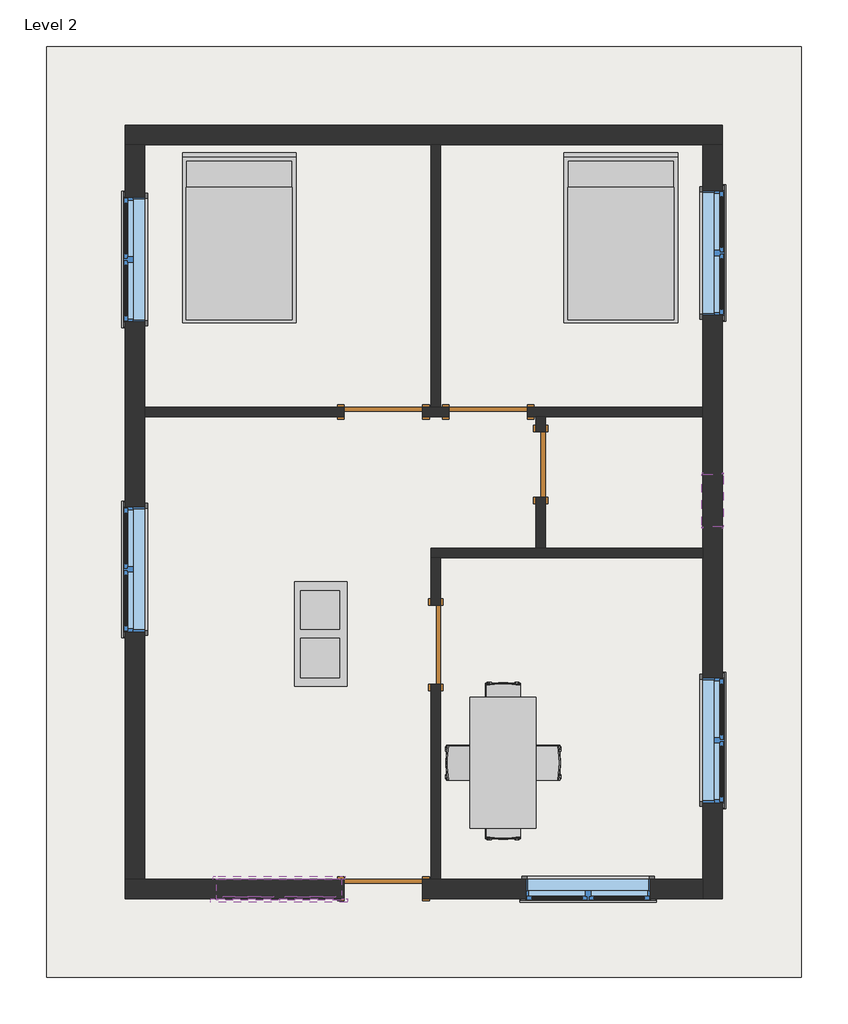
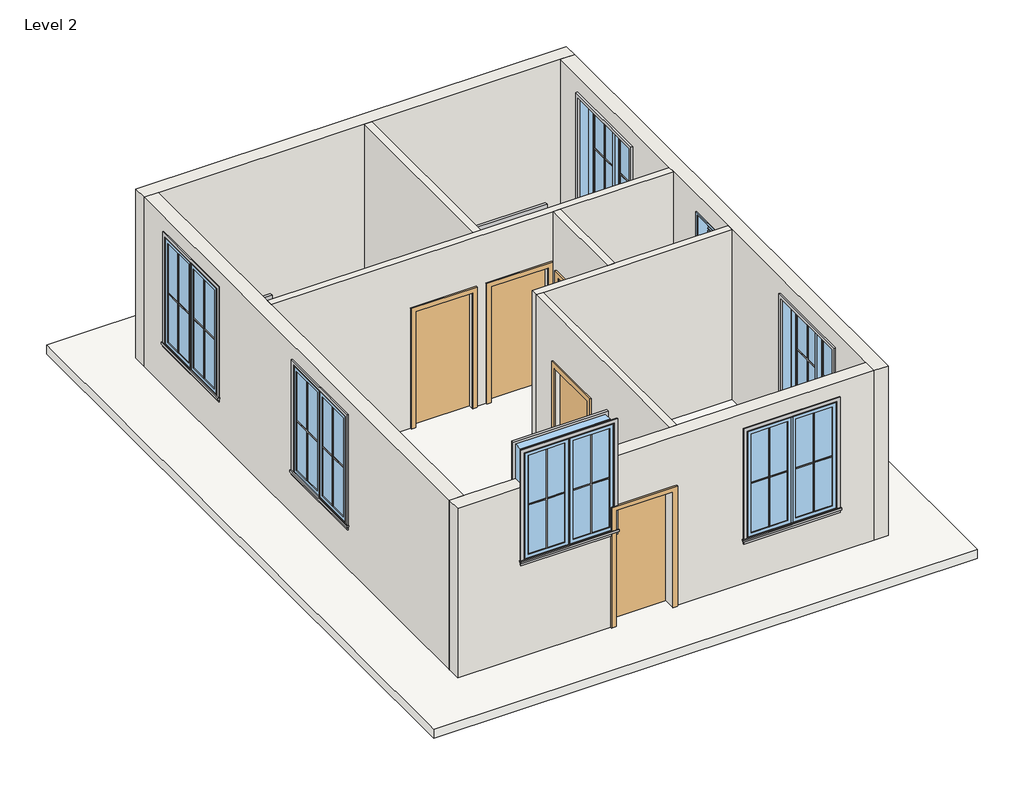
# One storey, incomplete: 25 proxies, 9 walls, 7 windows, 5 doors, 3 furniture elements, 1 roof.
"""IFC4 building model written with IfcOpenShell, lengths in millimetres."""

from ifc_helpers import new_model, si_unit, frame, origin, place, context, project, spatial, polyline, outline, extrude, faceted_brep, transform, mapped, element, save
from components import muntin_pattern_2x2_muntin_pattern_2x2_bff912c5, muntin_pattern_2x2_muntin_pattern_2x2_c2194282, trim_window_exterior_flat_with_sill_e04b3088, trim_window_interior_flat_picture_frame_2a7685fe, coffee_table_with_brass_mullions_11320_coffee_table_with_5962bef7, door_305aa2a5, door_e5f9f3c4, door_0ca8825f, door_f2b275c1, bed_17739_bed_17739_15c61121, dining_table_w_chairs_11374_0cdfc61b, window_9ac97e1a, window_f2d8fef0

model = new_model("IFC4")

# Units and contexts
model_context = context("Model", 3, world=origin())
ifc_project = project(units=[si_unit("LENGTHUNIT", "METRE", prefix="MILLI")], contexts=[model_context])

# Site, building, storey
site = spatial("IfcSite", under=ifc_project)
building = spatial("IfcBuilding", under=site)
storey = spatial("IfcBuildingStorey", under=building, Name="Level 2", Elevation=3048.0)

# Proxies
placement = place(None, origin())
muntin_pattern_2x2_muntin_pattern_2x2_shape = muntin_pattern_2x2_muntin_pattern_2x2_bff912c5(model_context)
element("IfcBuildingElementProxy", 1, Name="Muntin Pattern_2x2 : Muntin Pattern_2x2", ObjectType="Muntin Pattern_2x2 : Muntin Pattern_2x2", at=placement, inside=storey, context=model_context, shape_type="MappedRepresentation", body=[
    mapped(muntin_pattern_2x2_muntin_pattern_2x2_shape, transform((-4718.1437352, -1580.3188735, 4032.25), x_axis=(0.0, 1.0, 0.0), y_axis=(-1.0, 0.0, 0.0), z_axis=(0.0, 0.0, 1.0))),
])
element("IfcBuildingElementProxy", 2, Name="Muntin Pattern_2x2 : Muntin Pattern_2x2", ObjectType="Muntin Pattern_2x2 : Muntin Pattern_2x2", at=placement, inside=storey, context=model_context, shape_type="MappedRepresentation", body=[
    mapped(muntin_pattern_2x2_muntin_pattern_2x2_shape, transform((-2576.6062352, -5039.4813735, 4923.115521), x_axis=(-1.0, 0.0, 0.0), y_axis=(0.0, -1.0, 0.0), z_axis=(0.0, 0.0, 1.0))),
])
element("IfcBuildingElementProxy", 3, Name="Muntin Pattern_2x2 : Muntin Pattern_2x2", ObjectType="Muntin Pattern_2x2 : Muntin Pattern_2x2", at=placement, inside=storey, context=model_context, shape_type="MappedRepresentation", body=[
    mapped(muntin_pattern_2x2_muntin_pattern_2x2_shape, transform((1017.4937648, -5039.4813735, 4032.25), x_axis=(-1.0, 0.0, 0.0), y_axis=(0.0, -1.0, 0.0), z_axis=(0.0, 0.0, 1.0))),
])
element("IfcBuildingElementProxy", 4, Name="Muntin Pattern_2x2 : Muntin Pattern_2x2", ObjectType="Muntin Pattern_2x2 : Muntin Pattern_2x2", at=placement, inside=storey, context=model_context, shape_type="MappedRepresentation", body=[
    mapped(muntin_pattern_2x2_muntin_pattern_2x2_shape, transform((2209.7062648, -2847.1438735, 4032.25), x_axis=(0.0, -1.0, 0.0), y_axis=(1.0, 0.0, 0.0), z_axis=(0.0, 0.0, 1.0))),
])
element("IfcBuildingElementProxy", 5, Name="Muntin Pattern_2x2 : Muntin Pattern_2x2", ObjectType="Muntin Pattern_2x2 : Muntin Pattern_2x2", at=placement, inside=storey, context=model_context, shape_type="MappedRepresentation", body=[
    mapped(muntin_pattern_2x2_muntin_pattern_2x2_shape, transform((2209.7062648, 2817.0561265, 4032.25), x_axis=(0.0, -1.0, 0.0), y_axis=(1.0, 0.0, 0.0), z_axis=(0.0, 0.0, 1.0))),
])
element("IfcBuildingElementProxy", 6, Name="Muntin Pattern_2x2 : Muntin Pattern_2x2", ObjectType="Muntin Pattern_2x2 : Muntin Pattern_2x2", at=placement, inside=storey, context=model_context, shape_type="MappedRepresentation", body=[
    mapped(muntin_pattern_2x2_muntin_pattern_2x2_shape, transform((-4718.1437352, 2020.1311265, 4032.25), x_axis=(0.0, 1.0, 0.0), y_axis=(-1.0, 0.0, 0.0), z_axis=(0.0, 0.0, 1.0))),
])
muntin_pattern_2x2_muntin_pattern_2x2_2_shape = muntin_pattern_2x2_muntin_pattern_2x2_c2194282(model_context)
element("IfcBuildingElementProxy", 7, Name="Muntin Pattern_2x2 : Muntin Pattern_2x2", ObjectType="Muntin Pattern_2x2 : Muntin Pattern_2x2", at=placement, inside=storey, context=model_context, shape_type="MappedRepresentation", body=[
    mapped(muntin_pattern_2x2_muntin_pattern_2x2_2_shape, transform((-4718.1437352, -859.5938735, 4032.25), x_axis=(0.0, -1.0, 0.0), y_axis=(1.0, 0.0, 0.0), z_axis=(0.0, 0.0, 1.0))),
])
element("IfcBuildingElementProxy", 8, Name="Muntin Pattern_2x2 : Muntin Pattern_2x2", ObjectType="Muntin Pattern_2x2 : Muntin Pattern_2x2", at=placement, inside=storey, context=model_context, shape_type="MappedRepresentation", body=[
    mapped(muntin_pattern_2x2_muntin_pattern_2x2_2_shape, transform((-3297.3312352, -5039.4813735, 4923.115521), x_axis=(1.0, 0.0, 0.0), y_axis=(0.0, 1.0, 0.0), z_axis=(0.0, 0.0, 1.0))),
])
element("IfcBuildingElementProxy", 9, Name="Muntin Pattern_2x2 : Muntin Pattern_2x2", ObjectType="Muntin Pattern_2x2 : Muntin Pattern_2x2", at=placement, inside=storey, context=model_context, shape_type="MappedRepresentation", body=[
    mapped(muntin_pattern_2x2_muntin_pattern_2x2_2_shape, transform((296.7687648, -5039.4813735, 4032.25), x_axis=(1.0, 0.0, 0.0), y_axis=(0.0, 1.0, 0.0), z_axis=(0.0, 0.0, 1.0))),
])
element("IfcBuildingElementProxy", 10, Name="Muntin Pattern_2x2 : Muntin Pattern_2x2", ObjectType="Muntin Pattern_2x2 : Muntin Pattern_2x2", at=placement, inside=storey, context=model_context, shape_type="MappedRepresentation", body=[
    mapped(muntin_pattern_2x2_muntin_pattern_2x2_2_shape, transform((2209.7062648, -3567.8688735, 4032.25), x_axis=(0.0, 1.0, 0.0), y_axis=(-1.0, 0.0, 0.0), z_axis=(0.0, 0.0, 1.0))),
])
element("IfcBuildingElementProxy", 11, Name="Muntin Pattern_2x2 : Muntin Pattern_2x2", ObjectType="Muntin Pattern_2x2 : Muntin Pattern_2x2", at=placement, inside=storey, context=model_context, shape_type="MappedRepresentation", body=[
    mapped(muntin_pattern_2x2_muntin_pattern_2x2_2_shape, transform((2209.7062648, 2096.3311265, 4032.25), x_axis=(0.0, 1.0, 0.0), y_axis=(-1.0, 0.0, 0.0), z_axis=(0.0, 0.0, 1.0))),
])
element("IfcBuildingElementProxy", 12, Name="Muntin Pattern_2x2 : Muntin Pattern_2x2", ObjectType="Muntin Pattern_2x2 : Muntin Pattern_2x2", at=placement, inside=storey, context=model_context, shape_type="MappedRepresentation", body=[
    mapped(muntin_pattern_2x2_muntin_pattern_2x2_2_shape, transform((-4718.1437352, 2740.8561265, 4032.25), x_axis=(0.0, -1.0, 0.0), y_axis=(1.0, 0.0, 0.0), z_axis=(0.0, 0.0, 1.0))),
])
trim_window_exterior_flat_with_sill_shape = trim_window_exterior_flat_with_sill_e04b3088(model_context)
element("IfcBuildingElementProxy", 13, Name="Trim-Window-Exterior-Flat : with Sill", ObjectType="Trim-Window-Exterior-Flat : with Sill", at=placement, inside=storey, context=model_context, shape_type="MappedRepresentation", body=[
    mapped(trim_window_exterior_flat_with_sill_shape, transform((-4727.6687352, -1219.9563735, 5791.2), x_axis=(0.0, -1.0, 0.0), y_axis=(0.0, 0.0, 1.0), z_axis=(-1.0, 0.0, 0.0))),
])
element("IfcBuildingElementProxy", 14, Name="Trim-Window-Exterior-Flat : with Sill", ObjectType="Trim-Window-Exterior-Flat : with Sill", at=placement, inside=storey, context=model_context, shape_type="MappedRepresentation", body=[
    mapped(trim_window_exterior_flat_with_sill_shape, transform((-2936.9687352, -5049.0063735, 6682.065521), x_axis=(1.0, 0.0, 0.0), y_axis=(0.0, 0.0, 1.0), z_axis=(0.0, -1.0, 0.0))),
])
element("IfcBuildingElementProxy", 15, Name="Trim-Window-Exterior-Flat : with Sill", ObjectType="Trim-Window-Exterior-Flat : with Sill", at=placement, inside=storey, context=model_context, shape_type="MappedRepresentation", body=[
    mapped(trim_window_exterior_flat_with_sill_shape, transform((657.1312648, -5049.0063735, 5791.2), x_axis=(1.0, 0.0, 0.0), y_axis=(0.0, 0.0, 1.0), z_axis=(0.0, -1.0, 0.0))),
])
element("IfcBuildingElementProxy", 16, Name="Trim-Window-Exterior-Flat : with Sill", ObjectType="Trim-Window-Exterior-Flat : with Sill", at=placement, inside=storey, context=model_context, shape_type="MappedRepresentation", body=[
    mapped(trim_window_exterior_flat_with_sill_shape, transform((2219.2312648, -3207.5063735, 5791.2), x_axis=(0.0, 1.0, 0.0), y_axis=(0.0, 0.0, 1.0), z_axis=(1.0, 0.0, 0.0))),
])
element("IfcBuildingElementProxy", 17, Name="Trim-Window-Exterior-Flat : with Sill", ObjectType="Trim-Window-Exterior-Flat : with Sill", at=placement, inside=storey, context=model_context, shape_type="MappedRepresentation", body=[
    mapped(trim_window_exterior_flat_with_sill_shape, transform((2219.2312648, 2456.6936265, 5791.2), x_axis=(0.0, 1.0, 0.0), y_axis=(0.0, 0.0, 1.0), z_axis=(1.0, 0.0, 0.0))),
])
element("IfcBuildingElementProxy", 18, Name="Trim-Window-Exterior-Flat : with Sill", ObjectType="Trim-Window-Exterior-Flat : with Sill", at=placement, inside=storey, context=model_context, shape_type="MappedRepresentation", body=[
    mapped(trim_window_exterior_flat_with_sill_shape, transform((-4727.6687352, 2380.4936265, 5791.2), x_axis=(0.0, -1.0, 0.0), y_axis=(0.0, 0.0, 1.0), z_axis=(-1.0, 0.0, 0.0))),
])
trim_window_interior_flat_picture_frame_shape = trim_window_interior_flat_picture_frame_2a7685fe(model_context)
element("IfcBuildingElementProxy", 19, Name="Trim-Window-Interior-Flat : Picture Frame", ObjectType="Trim-Window-Interior-Flat : Picture Frame", at=placement, inside=storey, context=model_context, shape_type="MappedRepresentation", body=[
    mapped(trim_window_interior_flat_picture_frame_shape, transform((-4499.0687352, -1219.9563735, 5791.2), x_axis=(0.0, 1.0, 0.0), y_axis=(0.0, 0.0, 1.0), z_axis=(1.0, 0.0, 0.0))),
])
element("IfcBuildingElementProxy", 20, Name="Trim-Window-Interior-Flat : Picture Frame", ObjectType="Trim-Window-Interior-Flat : Picture Frame", at=placement, inside=storey, context=model_context, shape_type="MappedRepresentation", body=[
    mapped(trim_window_interior_flat_picture_frame_shape, transform((-2936.9687352, -4820.4063735, 6682.065521), x_axis=(-1.0, 0.0, 0.0), y_axis=(0.0, 0.0, 1.0), z_axis=(0.0, 1.0, 0.0))),
])
element("IfcBuildingElementProxy", 21, Name="Trim-Window-Interior-Flat : Picture Frame", ObjectType="Trim-Window-Interior-Flat : Picture Frame", at=placement, inside=storey, context=model_context, shape_type="MappedRepresentation", body=[
    mapped(trim_window_interior_flat_picture_frame_shape, transform((657.1312648, -4820.4063735, 5791.2), x_axis=(-1.0, 0.0, 0.0), y_axis=(0.0, 0.0, 1.0), z_axis=(0.0, 1.0, 0.0))),
])
element("IfcBuildingElementProxy", 22, Name="Trim-Window-Interior-Flat : Picture Frame", ObjectType="Trim-Window-Interior-Flat : Picture Frame", at=placement, inside=storey, context=model_context, shape_type="MappedRepresentation", body=[
    mapped(trim_window_interior_flat_picture_frame_shape, transform((1990.6312648, -3207.5063735, 5791.2), x_axis=(0.0, -1.0, 0.0), y_axis=(0.0, 0.0, 1.0), z_axis=(-1.0, 0.0, 0.0))),
])
element("IfcBuildingElementProxy", 23, Name="Trim-Window-Interior-Flat : Picture Frame", ObjectType="Trim-Window-Interior-Flat : Picture Frame", at=placement, inside=storey, context=model_context, shape_type="MappedRepresentation", body=[
    mapped(trim_window_interior_flat_picture_frame_shape, transform((1990.6312648, 2456.6936265, 5791.2), x_axis=(0.0, -1.0, 0.0), y_axis=(0.0, 0.0, 1.0), z_axis=(-1.0, 0.0, 0.0))),
])
element("IfcBuildingElementProxy", 24, Name="Trim-Window-Interior-Flat : Picture Frame", ObjectType="Trim-Window-Interior-Flat : Picture Frame", at=placement, inside=storey, context=model_context, shape_type="MappedRepresentation", body=[
    mapped(trim_window_interior_flat_picture_frame_shape, transform((-4499.0687352, 2380.4936265, 5791.2), x_axis=(0.0, 1.0, 0.0), y_axis=(0.0, 0.0, 1.0), z_axis=(1.0, 0.0, 0.0))),
])
coffee_table_with_brass_mullions_11320_coffee_table_with_shape = coffee_table_with_brass_mullions_11320_coffee_table_with_5962bef7(model_context)
element("IfcBuildingElementProxy", 25, Name="coffee_table_with_brass_mullions_11320 : coffee_table_with_brass_mullions_11320", ObjectType="coffee_table_with_brass_mullions_11320 : coffee_table_with_brass_mullions_11320", at=placement, inside=storey, context=model_context, shape_type="MappedRepresentation", body=[
    mapped(coffee_table_with_brass_mullions_11320_coffee_table_with_shape, transform((-2022.5687352, -1334.2563735, 3048.0), x_axis=(0.0, 1.0, 0.0), y_axis=(-1.0, 0.0, 0.0), z_axis=(0.0, 0.0, 1.0))),
])

# Doors
door_shape = door_305aa2a5(model_context)
element("IfcDoor", 26, ObjectType="Single-Flush : 36\" x 84\"", at=placement, inside=storey, context=model_context, shape_type="MappedRepresentation", body=[
    mapped(door_shape, transform((-1114.5187352, -2096.2563735, 3048.0), x_axis=(0.0, 1.0, 0.0), y_axis=(-1.0, 0.0, 0.0), z_axis=(0.0, 0.0, 1.0))),
])
element("IfcDoor", 27, ObjectType="Single-Flush : 36\" x 84\"", at=placement, inside=storey, context=model_context, shape_type="MappedRepresentation", body=[
    mapped(door_shape, transform((-1724.1187352, 608.8436265, 3048.0), x_axis=(-1.0, 0.0, 0.0), y_axis=(0.0, -1.0, 0.0), z_axis=(0.0, 0.0, 1.0))),
])
door_2_shape = door_e5f9f3c4(model_context)
element("IfcDoor", 28, ObjectType="Single-Flush : 36\" x 84\"", at=placement, inside=storey, context=model_context, shape_type="MappedRepresentation", body=[
    mapped(door_2_shape, transform((-504.9187352, 608.8436265, 3048.0), x_axis=(1.0, 0.0, 0.0), y_axis=(0.0, 1.0, 0.0), z_axis=(0.0, 0.0, 1.0))),
])
door_3_shape = door_0ca8825f(model_context)
element("IfcDoor", 29, ObjectType="Single-Flush : 36\" x 84\"", at=placement, inside=storey, context=model_context, shape_type="MappedRepresentation", body=[
    mapped(door_3_shape, transform((-1724.1187352, -4934.7063735, 3048.0), x_axis=(1.0, 0.0, 0.0), y_axis=(0.0, 1.0, 0.0), z_axis=(0.0, 0.0, 1.0))),
])
door_4_shape = door_f2b275c1(model_context)
element("IfcDoor", 30, ObjectType="Single-Flush : DOOR 2'6\"", at=placement, inside=storey, context=model_context, shape_type="MappedRepresentation", body=[
    mapped(door_4_shape, transform((104.6812648, -0.7563735, 3048.0), x_axis=(0.0, 1.0, 0.0), y_axis=(-1.0, 0.0, 0.0), z_axis=(0.0, 0.0, 1.0))),
])

# Furniture
bed_17739_bed_17739_shape = bed_17739_bed_17739_15c61121(model_context)
element("IfcFurniture", 31, ObjectType="Bed_17739 : Bed_17739", at=placement, inside=storey, context=model_context, shape_type="MappedRepresentation", body=[
    mapped(bed_17739_bed_17739_shape, transform((-3400.5187352, 2609.0936265, 3048.0), x_axis=(1.0, 0.0, 0.0), y_axis=(0.0, 1.0, 0.0), z_axis=(0.0, 0.0, 1.0))),
])
element("IfcFurniture", 32, ObjectType="Bed_17739 : Bed_17739", at=placement, inside=storey, context=model_context, shape_type="MappedRepresentation", body=[
    mapped(bed_17739_bed_17739_shape, transform((1038.1312648, 2609.0936265, 3048.0), x_axis=(1.0, 0.0, 0.0), y_axis=(0.0, 1.0, 0.0), z_axis=(0.0, 0.0, 1.0))),
])
dining_table_w_chairs_11374_shape = dining_table_w_chairs_11374_0cdfc61b(model_context)
element("IfcFurniture", 33, ObjectType="Dining_Table_w_Chairs_11374", at=placement, inside=storey, context=model_context, shape_type="MappedRepresentation", body=[
    mapped(dining_table_w_chairs_11374_shape, transform((-238.2576574, -3486.1221401, 3048.0), x_axis=(0.0, 1.0, 0.0), y_axis=(-1.0, 0.0, 0.0), z_axis=(0.0, 0.0, 1.0))),
])

# Roof
element("IfcRoof", 34, ObjectType="ROOF 6\"", at=placement, inside=storey, context=model_context, shape_type="SweptSolid", body=[
    extrude(outline(polyline([(-5642.0687352, 4856.9936265), (3133.6312648, 4856.9936265), (3133.6312648, -5963.4063735), (-5642.0687352, -5963.4063735), (-5642.0687352, 4856.9936265)])), frame((0.0, 0.0, 3048.0), z_axis=(0.0, 0.0, 1.0), x_axis=(1.0, 0.0, 0.0)), (0.0, 0.0, 1.0), 152.4),
])

# Walls
element("IfcWall", 35, ObjectType="WALL 4.5\"", at=placement, inside=storey, context=model_context, shape_type="Brep", body=[
    faceted_brep([(-4499.0687352, 551.6936265, 3048.0), (-2181.3187352, 551.6936265, 3048.0), (-2181.3187352, 551.6936265, 5181.6), (-1266.9187352, 551.6936265, 5181.6), (-1266.9187352, 551.6936265, 3048.0), (-962.1187352, 551.6936265, 3048.0), (-962.1187352, 551.6936265, 5181.6), (-47.7187352, 551.6936265, 5181.6), (-47.7187352, 551.6936265, 3048.0), (47.5312648, 551.6936265, 3048.0), (161.8312648, 551.6936265, 3048.0), (1990.6312648, 551.6936265, 3048.0), (1990.6312648, 551.6936265, 6096.0), (161.8312648, 551.6936265, 6096.0), (47.5312648, 551.6936265, 6096.0), (-4499.0687352, 551.6936265, 6096.0), (-2181.3187352, 665.9936265, 5181.6), (-2181.3187352, 665.9936265, 3048.0), (-4499.0687352, 665.9936265, 3048.0), (-4499.0687352, 665.9936265, 6096.0), (-1171.6687352, 665.9936265, 6096.0), (-1057.3687352, 665.9936265, 6096.0), (1990.6312648, 665.9936265, 6096.0), (1990.6312648, 665.9936265, 3048.0), (-47.7187352, 665.9936265, 3048.0), (-47.7187352, 665.9936265, 5181.6), (-962.1187352, 665.9936265, 5181.6), (-962.1187352, 665.9936265, 3048.0), (-1057.3687352, 665.9936265, 3048.0), (-1171.6687352, 665.9936265, 3048.0), (-1266.9187352, 665.9936265, 3048.0), (-1266.9187352, 665.9936265, 5181.6)], [[[0, 1, 2, 3, 4, 5, 6, 7, 8, 9, 10, 11, 12, 13, 14, 15]], [[16, 17, 18, 19, 20, 21, 22, 23, 24, 25, 26, 27, 28, 29, 30, 31]], [[11, 10, 9, 8, 24, 23]], [[18, 17, 1, 0]], [[30, 29, 28, 27, 5, 4]], [[12, 11, 23, 22]], [[0, 15, 19, 18]], [[25, 24, 8, 7]], [[26, 25, 7, 6]], [[27, 26, 6, 5]], [[2, 1, 17, 16]], [[3, 2, 16, 31]], [[4, 3, 31, 30]], [[15, 14, 13, 12, 22, 21, 20, 19]]]),
])
element("IfcWall", 36, ObjectType="WALL 4.5\"", at=placement, inside=storey, context=model_context, shape_type="SweptSolid", body=[
    extrude(outline(polyline([(-1057.3687352, 3713.9936265), (-1057.3687352, 665.9936265), (-1171.6687352, 665.9936265), (-1171.6687352, 3713.9936265), (-1057.3687352, 3713.9936265)])), frame((0.0, 0.0, 3048.0), z_axis=(0.0, 0.0, 1.0), x_axis=(1.0, 0.0, 0.0)), (0.0, 0.0, 1.0), 3048.0),
])
element("IfcWall", 37, ObjectType="WALL 4.5\"", at=placement, inside=storey, context=model_context, shape_type="Brep", body=[
    faceted_brep([(1990.6312648, -972.3063735, 3048.0), (161.8312648, -972.3063735, 3048.0), (47.5312648, -972.3063735, 3048.0), (-1171.6687352, -972.3063735, 3048.0), (-1171.6687352, -972.3063735, 6096.0), (47.5312648, -972.3063735, 6096.0), (161.8312648, -972.3063735, 6096.0), (1990.6312648, -972.3063735, 6096.0), (1990.6312648, -1086.6063735, 3048.0), (1990.6312648, -1086.6063735, 6096.0), (-1057.3687352, -1086.6063735, 6096.0), (-1171.6687352, -1086.6063735, 6096.0), (-1171.6687352, -1086.6063735, 3048.0), (-1057.3687352, -1086.6063735, 3048.0)], [[[0, 1, 2, 3, 4, 5, 6, 7]], [[8, 9, 10, 11, 12, 13]], [[3, 2, 1, 0, 8, 13, 12]], [[0, 7, 9, 8]], [[4, 3, 12, 11]], [[7, 6, 5, 4, 11, 10, 9]]]),
])
element("IfcWall", 38, ObjectType="WALL 4.5\"", at=placement, inside=storey, context=model_context, shape_type="SweptSolid", body=[
    extrude(outline(polyline([(-1086.6063735, 3048.0), (-1639.0563735, 3048.0), (-1639.0563735, 5181.6), (-2553.4563735, 5181.6), (-2553.4563735, 3048.0), (-4820.4063735, 3048.0), (-4820.4063735, 6096.0), (-1086.6063735, 6096.0), (-1086.6063735, 3048.0)])), frame((-1171.6687352, 0.0, 0.0), z_axis=(1.0, 0.0, 0.0), x_axis=(0.0, 1.0, 0.0)), (0.0, 0.0, 1.0), 114.3),
])
element("IfcWall", 39, ObjectType="WALL 4.5\"", at=placement, inside=storey, context=model_context, shape_type="SweptSolid", body=[
    extrude(outline(polyline([(551.6936265, 3048.0), (380.2436265, 3048.0), (380.2436265, 5080.0), (-381.7563735, 5080.0), (-381.7563735, 3048.0), (-972.3063735, 3048.0), (-972.3063735, 6096.0), (551.6936265, 6096.0), (551.6936265, 3048.0)])), frame((47.5312648, 0.0, 0.0), z_axis=(1.0, 0.0, 0.0), x_axis=(0.0, 1.0, 0.0)), (0.0, 0.0, 1.0), 114.3),
])
element("IfcWall", 40, ObjectType="WALL 9\"", at=placement, inside=storey, context=model_context, shape_type="Brep", body=[
    faceted_brep([(-4727.6687352, 3713.9936265, 3048.0), (-4499.0687352, 3713.9936265, 3048.0), (-1171.6687352, 3713.9936265, 3048.0), (-1057.3687352, 3713.9936265, 3048.0), (1990.6312648, 3713.9936265, 3048.0), (2219.2312648, 3713.9936265, 3048.0), (2219.2312648, 3713.9936265, 6096.0), (1990.6312648, 3713.9936265, 6096.0), (-1057.3687352, 3713.9936265, 6096.0), (-1171.6687352, 3713.9936265, 6096.0), (-4499.0687352, 3713.9936265, 6096.0), (-4727.6687352, 3713.9936265, 6096.0), (-4727.6687352, 3942.5936265, 3048.0), (-4727.6687352, 3942.5936265, 6096.0), (2219.2312648, 3942.5936265, 6096.0), (2219.2312648, 3942.5936265, 3048.0)], [[[0, 1, 2, 3, 4, 5, 6, 7, 8, 9, 10, 11]], [[12, 13, 14, 15]], [[5, 4, 3, 2, 1, 0, 12, 15]], [[6, 5, 15, 14]], [[0, 11, 13, 12]], [[11, 10, 9, 8, 7, 6, 14, 13]]]),
])
element("IfcWall", 41, ObjectType="WALL 9\"", at=placement, inside=storey, context=model_context, shape_type="Brep", body=[
    faceted_brep([(1990.6312648, 3713.9936265, 3048.0), (1990.6312648, 665.9936265, 3048.0), (1990.6312648, 551.6936265, 3048.0), (1990.6312648, -972.3063735, 3048.0), (1990.6312648, -1086.6063735, 3048.0), (1990.6312648, -4820.4063735, 3048.0), (1990.6312648, -5049.0063735, 3048.0), (1990.6312648, -5049.0063735, 6096.0), (1990.6312648, -4820.4063735, 6096.0), (1990.6312648, -1086.6063735, 6096.0), (1990.6312648, -972.3063735, 6096.0), (1990.6312648, 551.6936265, 6096.0), (1990.6312648, 665.9936265, 6096.0), (1990.6312648, 3713.9936265, 6096.0), (1990.6312648, -3931.4063735, 5791.2), (1990.6312648, -3931.4063735, 3962.4), (1990.6312648, -2483.6063735, 3962.4), (1990.6312648, -2483.6063735, 5791.2), (1990.6312648, 1732.7936265, 5791.2), (1990.6312648, 1732.7936265, 3962.4), (1990.6312648, 3180.5936265, 3962.4), (1990.6312648, 3180.5936265, 5791.2), (1990.6312648, -115.0563735, 5791.2), (1990.6312648, -724.6563735, 5791.2), (1990.6312648, -724.6563735, 5181.6), (1990.6312648, -115.0563735, 5181.6), (2219.2312648, 3713.9936265, 3048.0), (2219.2312648, 3713.9936265, 6096.0), (2219.2312648, -5049.0063735, 6096.0), (2219.2312648, -5049.0063735, 3048.0), (2219.2312648, -3931.4063735, 5791.2), (2219.2312648, -2483.6063735, 5791.2), (2219.2312648, -2483.6063735, 3962.4), (2219.2312648, -3931.4063735, 3962.4), (2219.2312648, 1732.7936265, 5791.2), (2219.2312648, 3180.5936265, 5791.2), (2219.2312648, 3180.5936265, 3962.4), (2219.2312648, 1732.7936265, 3962.4), (2219.2312648, -115.0563735, 5791.2), (2219.2312648, -115.0563735, 5181.6), (2219.2312648, -724.6563735, 5181.6), (2219.2312648, -724.6563735, 5791.2)], [[[0, 1, 2, 3, 4, 5, 6, 7, 8, 9, 10, 11, 12, 13], [14, 15, 16, 17], [18, 19, 20, 21], [22, 23, 24, 25]], [[26, 27, 28, 29], [30, 31, 32, 33], [34, 35, 36, 37], [38, 39, 40, 41]], [[6, 5, 4, 3, 2, 1, 0, 26, 29]], [[0, 13, 27, 26]], [[7, 6, 29, 28]], [[15, 14, 30, 33]], [[16, 15, 33, 32]], [[17, 16, 32, 31]], [[14, 17, 31, 30]], [[19, 18, 34, 37]], [[20, 19, 37, 36]], [[21, 20, 36, 35]], [[18, 21, 35, 34]], [[39, 38, 22, 25]], [[40, 39, 25, 24]], [[41, 40, 24, 23]], [[38, 41, 23, 22]], [[13, 12, 11, 10, 9, 8, 7, 28, 27]]]),
])
element("IfcWall", 42, ObjectType="WALL 9\"", at=placement, inside=storey, context=model_context, shape_type="Brep", body=[
    faceted_brep([(1990.6312648, -4820.4063735, 6096.0), (1990.6312648, -4820.4063735, 3048.0), (-1057.3687352, -4820.4063735, 3048.0), (-1171.6687352, -4820.4063735, 3048.0), (-1266.9187352, -4820.4063735, 3048.0), (-1266.9187352, -4820.4063735, 5181.6), (-2181.3187352, -4820.4063735, 5181.6), (-2181.3187352, -4820.4063735, 3048.0), (-4499.0687352, -4820.4063735, 3048.0), (-4727.6687352, -4820.4063735, 3048.0), (-4727.6687352, -4820.4063735, 6096.0), (-4499.0687352, -4820.4063735, 6096.0), (-3660.8687352, -4820.4063735, 6096.0), (-3660.8687352, -4820.4063735, 4853.265521), (-2213.0687352, -4820.4063735, 4853.265521), (-2213.0687352, -4820.4063735, 6096.0), (-1171.6687352, -4820.4063735, 6096.0), (-1057.3687352, -4820.4063735, 6096.0), (-66.7687352, -4820.4063735, 5791.2), (-66.7687352, -4820.4063735, 3962.4), (1381.0312648, -4820.4063735, 3962.4), (1381.0312648, -4820.4063735, 5791.2), (1990.6312648, -5049.0063735, 3048.0), (1990.6312648, -5049.0063735, 6096.0), (-2213.0687352, -5049.0063735, 6096.0), (-2213.0687352, -5049.0063735, 4853.265521), (-3660.8687352, -5049.0063735, 4853.265521), (-3660.8687352, -5049.0063735, 6096.0), (-4727.6687352, -5049.0063735, 6096.0), (-4727.6687352, -5049.0063735, 3048.0), (-2181.3187352, -5049.0063735, 3048.0), (-2181.3187352, -5049.0063735, 5181.6), (-1266.9187352, -5049.0063735, 5181.6), (-1266.9187352, -5049.0063735, 3048.0), (-66.7687352, -5049.0063735, 3962.4), (-66.7687352, -5049.0063735, 5791.2), (1381.0312648, -5049.0063735, 5791.2), (1381.0312648, -5049.0063735, 3962.4)], [[[0, 1, 2, 3, 4, 5, 6, 7, 8, 9, 10, 11, 12, 13, 14, 15, 16, 17], [18, 19, 20, 21]], [[22, 23, 24, 25, 26, 27, 28, 29, 30, 31, 32, 33], [34, 35, 36, 37]], [[1, 22, 33, 4, 3, 2]], [[29, 9, 8, 7, 30]], [[1, 0, 23, 22]], [[10, 9, 29, 28]], [[19, 18, 35, 34]], [[20, 19, 34, 37]], [[21, 20, 37, 36]], [[18, 21, 36, 35]], [[5, 4, 33, 32]], [[6, 5, 32, 31]], [[7, 6, 31, 30]], [[10, 28, 27, 12, 11]], [[23, 0, 17, 16, 15, 24]], [[26, 13, 12, 27]], [[13, 26, 25, 14]], [[14, 25, 24, 15]]]),
])
element("IfcWall", 43, ObjectType="WALL 9\"", at=placement, inside=storey, context=model_context, shape_type="Brep", body=[
    faceted_brep([(-4499.0687352, -4820.4063735, 3048.0), (-4499.0687352, 551.6936265, 3048.0), (-4499.0687352, 665.9936265, 3048.0), (-4499.0687352, 3713.9936265, 3048.0), (-4499.0687352, 3713.9936265, 6096.0), (-4499.0687352, 665.9936265, 6096.0), (-4499.0687352, 551.6936265, 6096.0), (-4499.0687352, -4820.4063735, 6096.0), (-4499.0687352, -496.0563735, 5791.2), (-4499.0687352, -496.0563735, 3962.4), (-4499.0687352, -1943.8563735, 3962.4), (-4499.0687352, -1943.8563735, 5791.2), (-4499.0687352, 3104.3936265, 5791.2), (-4499.0687352, 3104.3936265, 3962.4), (-4499.0687352, 1656.5936265, 3962.4), (-4499.0687352, 1656.5936265, 5791.2), (-4727.6687352, -4820.4063735, 3048.0), (-4727.6687352, -4820.4063735, 6096.0), (-4727.6687352, 3713.9936265, 6096.0), (-4727.6687352, 3713.9936265, 3048.0), (-4727.6687352, -496.0563735, 5791.2), (-4727.6687352, -1943.8563735, 5791.2), (-4727.6687352, -1943.8563735, 3962.4), (-4727.6687352, -496.0563735, 3962.4), (-4727.6687352, 3104.3936265, 5791.2), (-4727.6687352, 1656.5936265, 5791.2), (-4727.6687352, 1656.5936265, 3962.4), (-4727.6687352, 3104.3936265, 3962.4)], [[[0, 1, 2, 3, 4, 5, 6, 7], [8, 9, 10, 11], [12, 13, 14, 15]], [[16, 17, 18, 19], [20, 21, 22, 23], [24, 25, 26, 27]], [[3, 2, 1, 0, 16, 19]], [[4, 3, 19, 18]], [[0, 7, 17, 16]], [[9, 8, 20, 23]], [[10, 9, 23, 22]], [[11, 10, 22, 21]], [[8, 11, 21, 20]], [[13, 12, 24, 27]], [[14, 13, 27, 26]], [[15, 14, 26, 25]], [[12, 15, 25, 24]], [[7, 6, 5, 4, 18, 17]]]),
])

# Windows
window_shape = window_9ac97e1a(model_context)
element("IfcWindow", 44, ObjectType="Window-Casement-Double : 57\" x 72\"", at=placement, inside=storey, context=model_context, shape_type="MappedRepresentation", body=[
    mapped(window_shape, transform((-4613.3687352, -1219.9563735, 3048.0), x_axis=(0.0, 1.0, 0.0), y_axis=(-1.0, 0.0, 0.0), z_axis=(0.0, 0.0, 1.0))),
])
element("IfcWindow", 45, ObjectType="Window-Casement-Double : 57\" x 72\"", at=placement, inside=storey, context=model_context, shape_type="MappedRepresentation", body=[
    mapped(window_shape, transform((-2936.9687352, -4934.7063735, 3938.865521), x_axis=(-1.0, 0.0, 0.0), y_axis=(0.0, -1.0, 0.0), z_axis=(0.0, 0.0, 1.0))),
])
element("IfcWindow", 46, ObjectType="Window-Casement-Double : 57\" x 72\"", at=placement, inside=storey, context=model_context, shape_type="MappedRepresentation", body=[
    mapped(window_shape, transform((657.1312648, -4934.7063735, 3048.0), x_axis=(-1.0, 0.0, 0.0), y_axis=(0.0, -1.0, 0.0), z_axis=(0.0, 0.0, 1.0))),
])
element("IfcWindow", 47, ObjectType="Window-Casement-Double : 57\" x 72\"", at=placement, inside=storey, context=model_context, shape_type="MappedRepresentation", body=[
    mapped(window_shape, transform((2104.9312648, -3207.5063735, 3048.0), x_axis=(0.0, -1.0, 0.0), y_axis=(1.0, 0.0, 0.0), z_axis=(0.0, 0.0, 1.0))),
])
element("IfcWindow", 48, ObjectType="Window-Casement-Double : 57\" x 72\"", at=placement, inside=storey, context=model_context, shape_type="MappedRepresentation", body=[
    mapped(window_shape, transform((2104.9312648, 2456.6936265, 3048.0), x_axis=(0.0, -1.0, 0.0), y_axis=(1.0, 0.0, 0.0), z_axis=(0.0, 0.0, 1.0))),
])
element("IfcWindow", 49, ObjectType="Window-Casement-Double : 57\" x 72\"", at=placement, inside=storey, context=model_context, shape_type="MappedRepresentation", body=[
    mapped(window_shape, transform((-4613.3687352, 2380.4936265, 3048.0), x_axis=(0.0, 1.0, 0.0), y_axis=(-1.0, 0.0, 0.0), z_axis=(0.0, 0.0, 1.0))),
])
window_2_shape = window_f2d8fef0(model_context)
element("IfcWindow", 50, ObjectType="Window-Louvers : 24\" x 24\"", at=placement, inside=storey, context=model_context, shape_type="MappedRepresentation", body=[
    mapped(window_2_shape, transform((2111.2812648, -419.8563735, 4267.2), x_axis=(0.0, -1.0, 0.0), y_axis=(1.0, 0.0, 0.0), z_axis=(0.0, 0.0, 1.0))),
])

save(model, "model.ifc")

# Revit data of these elements
# Type "Muntin Pattern_2x2 : Muntin Pattern_2x2"
#   Width [instance default] = 4' - 0"
#   Thickness = 0' - 0 1/2"
#   Height [instance default] = 4' - 0"
#   Distance = 0' - 0 3/4"
#   Interior Material [instance default] = none
#   Exterior Material [instance default] = none
#   Default Elevation = 0
# Type "Trim-Window-Exterior-Flat : with Sill"
#   Trim Width = 0' - 2 1/4"
#   Trim Thickness_Picture Frame = 0' - 1 1/4"
#   Trim Thickness_with Sill = 0' - 0 3/4"
#   Sill Thickness = 0' - 1 1/4"
#   Opening Width [instance default] = 2' - 0"
#   Opening Height [instance default] = 3' - 0"
#   Default Elevation = 4' - 0"
#   Sill = yes
#   Picture Frame = no
#   Trim Material [instance default] = none
# Type "Trim-Window-Interior-Flat : Picture Frame"
#   Trim Thickness_Picture Frame = 0' - 1 1/4"
#   Trim Width = 0' - 2 1/4"
#   Trim Thickness_with Sill = 0' - 0 3/4"
#   Sill Thickness = 0' - 1 1/4"
#   Opening Width [instance default] = 2' - 0"
#   Opening Height [instance default] = 3' - 0"
#   Default Elevation = 4' - 0"
#   Sill = no
#   Picture Frame = yes
#   Trim Material [instance default] = none
# Type "coffee_table_with_brass_mullions_11320 : coffee_table_with_brass_mullions_11320"
#   Default Elevation = 0
# Type "Single-Flush : 36\" x 84\""
#   Type Mark = "1"
#   Construction Type Id = "MDOOR"
#   Assembly Code = "C1020"
#   Analytic Construction = "Metal"
#   Thickness = 0' - 2"
#   Heat Transfer Coefficient (U) = 0.651978 BTU/(h·ft²·°F)
#   Height = 7' - 0"
#   Trim Projection Ext = 0' - 1"
#   Trim Projection Int = 0' - 1"
#   Trim Width = 0' - 3"
#   Width = 3' - 0"
#   Define Thermal Properties by = 1
#   Define Thermal Properties by = 1
#   Door Material = Door - Panel
#   Frame Material = Door - Frame
#   Visual Light Transmittance = 0
#   Solar Heat Gain Coefficient = 0
#   Function = (empty or 0)
#   Wall Closure = (empty or 0)
# Type "Single-Flush : DOOR 2'6\""
#   Type Mark = "8"
#   Construction Type Id = "MDOOR"
#   Assembly Code = "C1020"
#   Analytic Construction = "Metal"
#   Thickness = 0' - 2"
#   Heat Transfer Coefficient (U) = 0.651978 BTU/(h·ft²·°F)
#   Height = 6' - 8"
#   Trim Projection Ext = 0' - 1"
#   Trim Projection Int = 0' - 1"
#   Trim Width = 0' - 3"
#   Width = 2' - 6"
#   Define Thermal Properties by = 1
#   Door Material = Door - Panel
#   Frame Material = Door - Frame
#   Visual Light Transmittance = 0
#   Solar Heat Gain Coefficient = 0
#   Function = (empty or 0)
#   Wall Closure = (empty or 0)
# Type "Bed_17739 : Bed_17739"
#   Default Elevation = 0
# Type "Dining_Table_w_Chairs_11374"
#   Default Elevation = 0
#   Assembly Code = ""
# Type "ROOF 6\""
#   Assembly Code = "B1020"
#   Layers, outside or top first: 0' - 6" no material (function 1)
# Type "WALL 4.5\""
#   Assembly Code = "B2010"
#   Layers, outside or top first: 0' - 4 1/2" no material (function 1)
# Type "WALL 9\""
#   Assembly Code = "B2010"
#   Layers, outside or top first: 0' - 9" no material (function 1)
# Type "Window-Casement-Double : 57\" x 72\""
#   Type Mark = "17"
#   Fire Rating = "0.5h"
#   Assembly Code = "B2020100"
#   Analytic Construction = "Double glazing - domestic"
#   Frame Extension [instance default] = 0' - 0 1/4"
#   Window Inset [instance default] = 0' - 0"
#   Wall Thickness [instance default] = 0' - 6"
#   Interior Wall Closure [instance default] = 0' - 2 1/4"
#   Half Width = 2' - 4 1/2"
#   Visual Light Transmittance = 0.81
#   Thermal Resistance (R) = 1.8146 (h·ft²·°F)/BTU
#   Solar Heat Gain Coefficient = 0.76
#   Rough Width = 4' - 9 1/2"
#   Rough Height = 6' - 0 1/2"
#   Height = 6' - 0"
#   Heat Transfer Coefficient (U) = 0.5511 BTU/(h·ft²·°F)
#   Exterior Wall Closure [instance default] = 0' - 1 1/4"
#   Extension Jamb [instance default] = 0' - 2 1/4"
#   Default Sill Height = 3' - 0"
#   Width = 4' - 9"
#   Define Thermal Properties by = 0
#   Muntin Visibility = yes
#   Interior Trim Visibility [instance default] = yes
#   Exterior Trim Visibility [instance default] = yes
#   Extension Jamb Visibility [instance default] = yes
#   Interior Trim Material = Wood - Stained
#   Muntin Pattern = Muntin Pattern_2x2 : Muntin Pattern_2x2
#   Interior Trim = Trim-Window-Interior-Flat : Picture Frame
#   Interior Frame Material = Wood - Stained
#   Glass Panel Material = Glass
#   Exterior Trim Material = Clad - White
#   Exterior Trim = Trim-Window-Exterior-Flat : with Sill
#   Exterior Frame Material = Clad - White
#   Wall Closure = (empty or 0)
# Type "Window-Louvers : 24\" x 24\""
#   Type Mark = "18"
#   Construction Type Id = "GSP4R"
#   Assembly Code = "B20"
#   Analytic Construction = "1/8 in Pilkington single glazing"
#   Visual Light Transmittance = 0.9
#   Thermal Resistance (R) = 1.53941 (h·ft²·°F)/BTU
#   Solar Heat Gain Coefficient = 0.78
#   Max Height = 1' - 11.74264"
#   Height = 2' - 0"
#   Heat Transfer Coefficient (U) = 0.6496 BTU/(h·ft²·°F)
#   Blade Width [instance default] = 1' - 10 1/2"
#   Blade Vertical Thickness = 0' - 0.35355"
#   Blade Thickness = 0' - 0 1/4"
#   Blade Spacing = 0' - 1 1/2"
#   Blade Height = 0' - 1.85355"
#   Blade Depth = 0' - 3"
#   Blade Angle = 45.00°
#   Default Sill Height = 3' - 0"
#   Trim Projection_Exterior = 0' - 0 1/2"
#   Trim Projection_Interior = 0' - 0 1/2"
#   Trim Width_Exterior = 0' - 1 1/2"
#   Trim Width_Interior = 0' - 1 1/2"
#   Width = 2' - 0"
#   Max Blade Count = 12
#   Define Thermal Properties by = 1
#   Blade Count = 12
#   Frame Material = Birch
#   Louver Material = Birch
#   Trim Exterior Material = Birch
#   Trim Interior Material = Birch
#   Wall Closure = (empty or 0)
# Elements 1, 2, 3, 4, 5, 6, 7, 8, 9, 10, 11, 12 (IfcBuildingElementProxy, "Muntin Pattern_2x2 : Muntin Pattern_2x2")
#   Width = 1' - 11 1/8"
#   Height = 5' - 6 1/2"
#   Interior Material = Wood - Stained
#   Exterior Material = Clad - White
#   Phase Created = New Construction
#   Materials on its faces: "Clad - White", "Wood - Stained"
# Elements 13, 14, 15, 16, 17, 18 (IfcBuildingElementProxy, "Trim-Window-Exterior-Flat : with Sill")
#   Opening Width = 4' - 9"
#   Opening Height = 6' - 0"
#   Trim Material = Clad - White
#   Phase Created = New Construction
#   Materials on its faces: "Clad - White"
# Elements 19, 20, 21, 22, 23, 24 (IfcBuildingElementProxy, "Trim-Window-Interior-Flat : Picture Frame")
#   Opening Width = 4' - 9"
#   Opening Height = 6' - 0"
#   Trim Material = Wood - Stained
#   Phase Created = New Construction
#   Materials on its faces: "Wood - Stained"
# Element 25 (IfcBuildingElementProxy, "coffee_table_with_brass_mullions_11320 : coffee_table_with_brass_mullions_11320")
#   Phase Created = New Construction
#   Materials on its faces: "Default Wall", "TABLE", "Glass", "Default"
# Elements 26, 27, 28, 29 (IfcDoor, "Single-Flush : 36\" x 84\"")
#   Phase Created = New Construction
#   Materials on its faces: "Door - Frame", "Door - Panel"
# Element 30 (IfcDoor, "Single-Flush : DOOR 2'6\"")
#   Phase Created = New Construction
#   Materials on its faces: "Door - Frame", "Door - Panel"
# Elements 31, 32 (IfcFurniture, "Bed_17739 : Bed_17739")
#   Phase Created = New Construction
#   Materials on its faces: "legs", "sheets", "bed frame", "Blanket"
# Element 33 (IfcFurniture, "Dining_Table_w_Chairs_11374")
#   Phase Created = New Construction
# Element 34 (IfcRoof, "ROOF 6\"")
#   built-in parameter 1001705 = 10.5 (stored number, unit not read)
#   built-in parameter 1001710 = 33615
#   Phase Created = New Construction
#   Materials on its faces: "Copper", "Default Roof", "Wood - Stained"
# Elements 35, 36, 37, 38, 39 (IfcWall, "WALL 4.5\"")
#   Top Offset = 0' - 0"
#   Base Offset = 0' - 0"
#   Unconnected Height = 10' - 0"
#   wall height = 10' - 0"
#   Phase Created = New Construction
#   Base Constraint = Level 2
#   Materials on its faces: "Default Wall"
# Elements 40, 41, 42, 43 (IfcWall, "WALL 9\"")
#   Top Offset = 0' - 0"
#   Base Offset = 0' - 0"
#   Unconnected Height = 10' - 0"
#   wall height = 10' - 0"
#   Phase Created = New Construction
#   Base Constraint = Level 2
#   Materials on its faces: "Default Wall", "Parking Stripe"
# Element 44 (IfcWindow, "Window-Casement-Double : 57\" x 72\"")
#   Mark = "8"
#   Window Inset = 0' - 0"
#   Interior Wall Closure = 0' - 2 1/4"
#   Frame Extension = 0' - 0 1/4"
#   Exterior Wall Closure = 0' - 1 1/4"
#   Interior Trim Visibility = yes
#   Exterior Trim Visibility = yes
#   Phase Created = New Construction
#   Materials on its faces: "Wood - Stained", "Glass", "Clad - White"
# Element 45 (IfcWindow, "Window-Casement-Double : 57\" x 72\"")
#   Mark = "9"
#   Window Inset = 0' - 0"
#   Interior Wall Closure = 0' - 2 1/4"
#   Frame Extension = 0' - 0 1/4"
#   Exterior Wall Closure = 0' - 1 1/4"
#   Interior Trim Visibility = yes
#   Exterior Trim Visibility = yes
#   Phase Created = New Construction
#   Materials on its faces: "Wood - Stained", "Glass", "Clad - White"
# Element 46 (IfcWindow, "Window-Casement-Double : 57\" x 72\"")
#   Mark = "10"
#   Window Inset = 0' - 0"
#   Interior Wall Closure = 0' - 2 1/4"
#   Frame Extension = 0' - 0 1/4"
#   Exterior Wall Closure = 0' - 1 1/4"
#   Interior Trim Visibility = yes
#   Exterior Trim Visibility = yes
#   Phase Created = New Construction
#   Materials on its faces: "Wood - Stained", "Glass", "Clad - White"
# Element 47 (IfcWindow, "Window-Casement-Double : 57\" x 72\"")
#   Mark = "11"
#   Window Inset = 0' - 0"
#   Interior Wall Closure = 0' - 2 1/4"
#   Frame Extension = 0' - 0 1/4"
#   Exterior Wall Closure = 0' - 1 1/4"
#   Interior Trim Visibility = yes
#   Exterior Trim Visibility = yes
#   Phase Created = New Construction
#   Materials on its faces: "Wood - Stained", "Glass", "Clad - White"
# Element 48 (IfcWindow, "Window-Casement-Double : 57\" x 72\"")
#   Mark = "12"
#   Window Inset = 0' - 0"
#   Interior Wall Closure = 0' - 2 1/4"
#   Frame Extension = 0' - 0 1/4"
#   Exterior Wall Closure = 0' - 1 1/4"
#   Interior Trim Visibility = yes
#   Exterior Trim Visibility = yes
#   Phase Created = New Construction
#   Materials on its faces: "Wood - Stained", "Glass", "Clad - White"
# Element 49 (IfcWindow, "Window-Casement-Double : 57\" x 72\"")
#   Mark = "13"
#   Window Inset = 0' - 0"
#   Interior Wall Closure = 0' - 2 1/4"
#   Frame Extension = 0' - 0 1/4"
#   Exterior Wall Closure = 0' - 1 1/4"
#   Interior Trim Visibility = yes
#   Exterior Trim Visibility = yes
#   Phase Created = New Construction
#   Materials on its faces: "Wood - Stained", "Glass", "Clad - White"
# Element 50 (IfcWindow, "Window-Louvers : 24\" x 24\"")
#   Mark = "14"
#   Blade Width = 1' - 10 1/2"
#   Phase Created = New Construction
#   Materials on its faces: "Birch"
# Materials
#   "Door - Panel": class "Wood", colour RGB 210 159 95, transparency 0, Cost = 0
#   "Door - Frame": colour RGB 118 70 51, transparency 0, Cost = 0
#   "Wood - Stained": class "Wood", colour RGB 224 178 126, transparency 0, Cost = 0
#   "Glass": class "Glass", colour RGB 0 128 192, transparency 0.75, Description = "Soda Lime Glass", Cost = 0
#   "Clad - White": class "Wood", colour RGB 242 242 238, transparency 0, Cost = 0
#   "Birch": class "Wood", colour RGB 224 178 126, transparency 0, Description = "Betula Alleghaniensis", Cost = 0
#   "Default Wall": colour RGB 128 128 128, transparency 0, Cost = 0
#   "TABLE": class "Generic", colour RGB 120 120 120, transparency 0, Cost = 0
#   "Default": colour RGB 127 127 127, transparency 0, Cost = 0
#   "legs": colour RGB 90 73 37, transparency 0, Cost = 0
#   "sheets": colour RGB 200 195 176, transparency 0, Cost = 0
#   "bed frame": colour RGB 90 73 37, transparency 0, Cost = 0
#   "Blanket": class "System", colour RGB 59 0 1, transparency 0, Cost = 0
#   "Copper": class "Metal", colour RGB 0 0 0, transparency 0, Description = "Copper, matte finish", Cost = 0
#   "Default Roof": colour RGB 88 101 114, transparency 0, Cost = 0
#   "Parking Stripe": class "Paint", colour RGB 250 250 91, transparency 0, Cost = 0
